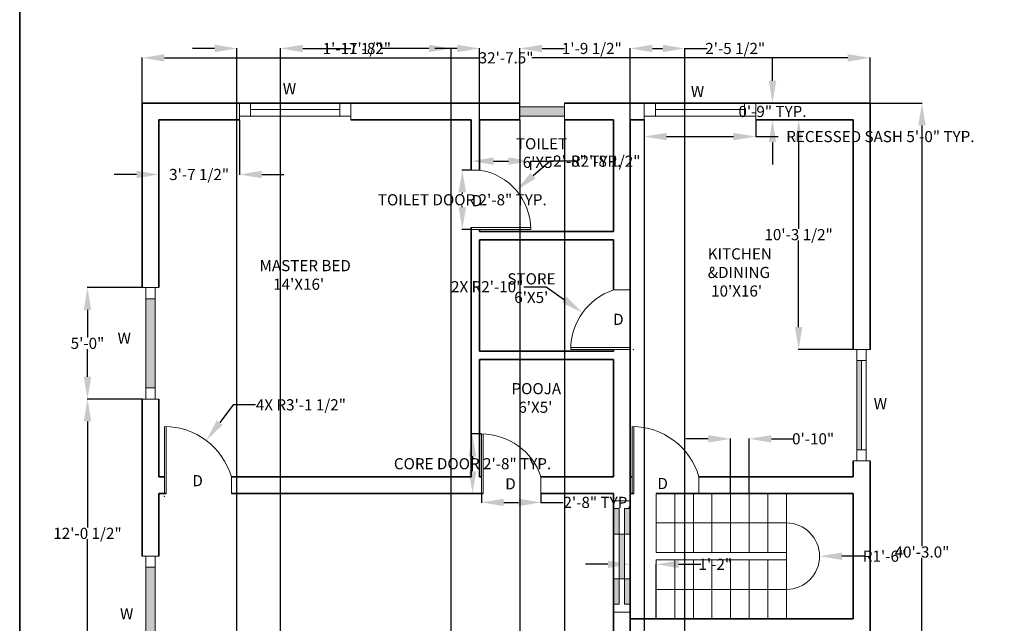
# Model space of a CAD drawing. Units: inches. Extents: x 115 to 1174, y 222 to 1302.
# Tile 2 of 5: x 115 to 644, y 521 to 846. Entities that reach past the tile are written whole.
import ezdxf

# ---------------------------------------------------------------- set-up
doc = ezdxf.new("R2010")
doc.units = ezdxf.units.IN
doc.header["$MEASUREMENT"] = 0
for name, color, linetype, lineweight in [('A-ANNO-DIMS', 2, 'Continuous', 18), ('A-ANNO-IDEN', 7, 'Continuous', 13), ('A-ANNO-TTLB', 7, 'Continuous', 35), ('A-AREA-IDEN', 7, 'Continuous', 18), ('A-DOOR', 3, 'Continuous', 18), ('A-FLOR-STRS', 7, 'Continuous', 18), ('A-GLAZ', 4, 'Continuous', 18), ('A-GLAZ-PATT', 8, 'Continuous', 13), ('A-WALL', 7, 'Continuous', 35)]:
    doc.layers.add(name, color=color, linetype=linetype, lineweight=lineweight)
doc.styles.get("Standard").update_dxf_attribs({"font": 'arial.ttf'})
doc.dimstyles.get("Standard").update_dxf_attribs({"dimtxt": 6, "dimasz": 12, "dimexe": 0.18, "dimexo": 0.0625, "dimgap": 0.09, "dimtad": 0, "dimtih": 1, "dimtoh": 1, "dimdec": 1, "dimzin": 0, "dimdsep": 46, "dimlunit": 3, "dimtxsty": 'Standard', "dimcen": 0.09, "dimadec": 0, "dimazin": 0, "dimtfac": 1, "dimtdec": 1, "dimtofl": 0, "dimtmove": 0, "dimatfit": 3, "dimfxl": 1, "dimtolj": 1, "dimtzin": 0, "dimarcsym": 0})

# ---------------------------------------------------------------- blocks, each defined once
blk = doc.blocks.new('*D1')
at = {"layer": 'A-ANNO-DIMS', "color": 0, "lineweight": -2, "transparency": 16777216}
for p, q in [((180.72, 801.13), (180.72, 825.59)), ((192.72, 825.41), (362.58, 825.41)), ((560.22, 825.41), (390.36, 825.41)), ((572.22, 801.13), (572.22, 825.59))]:
    blk.add_line(p, q, dxfattribs=at)
at = {"layer": 'A-ANNO-DIMS', "color": 0, "transparency": 16777216}
for points in [[(192.72, 827.41), (192.72, 823.41), (180.72, 825.41)], [(560.22, 827.41), (560.22, 823.41), (572.22, 825.41)]]:
    blk.add_solid(points, dxfattribs=at)
at = {"layer": 'Defpoints', "color": 0, "transparency": 16777216}
for p in [(572.22, 825.41), (180.72, 801.06), (572.22, 801.06)]:
    blk.add_point(p, dxfattribs=at)
at = {"layer": 'A-ANNO-DIMS', "color": 0, "transparency": 16777216, "insert": (376.47, 825.41), "char_height": 6, "attachment_point": 5}
blk.add_mtext('\\A1;32\'-7.5"', dxfattribs=at)
blk = doc.blocks.new('*D2')
at = {"layer": 'A-ANNO-DIMS', "color": 0, "lineweight": -2, "transparency": 16777216}
for p, q in [((572.28, 801.06), (600.35, 801.06)), ((600.17, 789.06), (600.17, 562.72)), ((600.17, 330.06), (600.17, 556.41)), ((572.28, 318.06), (600.35, 318.06))]:
    blk.add_line(p, q, dxfattribs=at)
at = {"layer": 'A-ANNO-DIMS', "color": 0, "transparency": 16777216}
for points in [[(598.17, 789.06), (602.17, 789.06), (600.17, 801.06)], [(598.17, 330.06), (602.17, 330.06), (600.17, 318.06)]]:
    blk.add_solid(points, dxfattribs=at)
at = {"layer": 'Defpoints', "color": 0, "transparency": 16777216}
for p in [(572.22, 801.06), (572.22, 318.06), (600.17, 318.06)]:
    blk.add_point(p, dxfattribs=at)
at = {"layer": 'A-ANNO-DIMS', "color": 0, "transparency": 16777216, "insert": (600.17, 559.56), "char_height": 6, "attachment_point": 5}
blk.add_mtext('\\A1;40\'-3.0"', dxfattribs=at)
blk = doc.blocks.new('DOOR-36-SWING')
for p, q in [((0, 0), (0, 36)), ((0, 36), (0, 0)), ((1, 36), (1, 0)), ((36, 0), (36, 9)), ((0, 0), (1, 0))]:
    blk.add_line(p, q)
blk.add_arc((0, -1.5), 37.5, 16.2602, 90)
blk = doc.blocks.new('DOOR-32-SWING')
for p, q in [((32, 32), (23, 32)), ((0, 1), (32, 1)), ((32, 0), (0, 0)), ((0, 0), (32, 0)), ((32, 0), (32, 1))]:
    blk.add_line(p, q)
blk.add_arc((33.76, 0), 33.76, 108.5866, 180)
blk = doc.blocks.new('DOOR-32-PARTITION')
for p, q in [((0, 32), (4.5, 32)), ((0, 0), (0, 1)), ((32, 1), (0, 1)), ((0, 0), (32, 0)), ((32, 0), (0, 0))]:
    blk.add_line(p, q)
blk.add_arc((-0.37, 0), 32.37, 0, 81.3499)
blk = doc.blocks.new('STAIR-HALF-TURN')
for p, q in [((0, 67.5), (0, 35.75)), ((10, 67.5), (10, 35.75)), ((20, 67.5), (20, 35.75)), ((30, 67.5), (30, 35.75)), ((40, 67.5), (40, 35.75)), ((50, 67.5), (50, 35.75)), ((60, 67.5), (60, 35.75)), ((70, 67.5), (70, 0)), ((106, 67.5), (106, 0)), ((0, 51.63), (70, 51.63)), ((70, 35.75), (0, 35.75)), ((70, 31.75), (0, 31.75)), ((0, 31.75), (0, 0)), ((10, 31.75), (10, 0)), ((20, 31.75), (20, 0)), ((30, 31.75), (30, 0)), ((40, 31.75), (40, 0)), ((50, 31.75), (50, 0)), ((60, 31.75), (60, 0)), ((0, 15.88), (70, 15.88))]:
    blk.add_line(p, q)
blk.add_arc((70, 33.75), 17.88, 270, 90)
blk = doc.blocks.new('WIN-60-RECESSED')
for p, q in [((0, 9), (0, 0)), ((60, 9), (0, 9)), ((6, 9), (6, 2)), ((6, 5.5), (54, 5.5)), ((54, 2), (54, 9)), ((60, 0), (60, 9)), ((0, 2), (60, 2))]:
    blk.add_line(p, q)
blk = doc.blocks.new('*D19')
at = {"layer": 'A-ANNO-DIMS', "color": 0, "lineweight": -2, "transparency": 16777216}
for p, q in [((363.16, 623.06), (358.24, 623.06)), ((358.42, 611.06), (358.42, 610.26)), ((358.42, 603.06), (358.42, 603.87)), ((363.16, 591.06), (358.24, 591.06))]:
    blk.add_line(p, q, dxfattribs=at)
at = {"layer": 'A-ANNO-DIMS', "color": 0, "transparency": 16777216}
for points in [[(356.42, 611.06), (360.42, 611.06), (358.42, 623.06)], [(356.42, 603.06), (360.42, 603.06), (358.42, 591.06)]]:
    blk.add_solid(points, dxfattribs=at)
at = {"layer": 'Defpoints', "color": 0, "transparency": 16777216}
for p in [(363.22, 623.06), (358.42, 591.06), (363.22, 591.06)]:
    blk.add_point(p, dxfattribs=at)
at = {"layer": 'A-ANNO-DIMS', "color": 0, "transparency": 16777216, "insert": (358.42, 607.06), "char_height": 6, "attachment_point": 5}
blk.add_mtext('\\A1;CORE DOOR 2\'-8" TYP.', dxfattribs=at)
blk = doc.blocks.new('*D20')
at = {"layer": 'A-ANNO-DIMS', "color": 0, "lineweight": -2, "transparency": 16777216}
for p, q in [((363.22, 591), (363.22, 586.08)), ((395.22, 591), (395.22, 586.08)), ((375.22, 586.26), (383.22, 586.26)), ((395.22, 586.26), (407.22, 586.26))]:
    blk.add_line(p, q, dxfattribs=at)
at = {"layer": 'A-ANNO-DIMS', "color": 0, "transparency": 16777216}
for points in [[(375.22, 588.26), (375.22, 584.26), (363.22, 586.26)], [(383.22, 588.26), (383.22, 584.26), (395.22, 586.26)]]:
    blk.add_solid(points, dxfattribs=at)
at = {"layer": 'Defpoints', "color": 0, "transparency": 16777216}
for p in [(363.22, 591.06), (395.22, 591.06), (395.22, 586.26)]:
    blk.add_point(p, dxfattribs=at)
at = {"layer": 'A-ANNO-DIMS', "color": 0, "transparency": 16777216, "insert": (425.65, 586.26), "char_height": 6, "attachment_point": 5}
blk.add_mtext('\\A1;2\'-8" TYP.', dxfattribs=at)
blk = doc.blocks.new('*D21')
at = {"layer": 'A-ANNO-DIMS', "color": 0, "lineweight": -2, "transparency": 16777216}
for p, q in [((357.66, 765.06), (352.74, 765.06)), ((352.92, 753.06), (352.92, 752.26)), ((352.92, 745.06), (352.92, 745.87)), ((357.66, 733.06), (352.74, 733.06))]:
    blk.add_line(p, q, dxfattribs=at)
at = {"layer": 'A-ANNO-DIMS', "color": 0, "transparency": 16777216}
for points in [[(350.92, 753.06), (354.92, 753.06), (352.92, 765.06)], [(350.92, 745.06), (354.92, 745.06), (352.92, 733.06)]]:
    blk.add_solid(points, dxfattribs=at)
at = {"layer": 'Defpoints', "color": 0, "transparency": 16777216}
for p in [(352.92, 765.06), (357.72, 765.06), (357.72, 733.06)]:
    blk.add_point(p, dxfattribs=at)
at = {"layer": 'A-ANNO-DIMS', "color": 0, "transparency": 16777216, "insert": (352.92, 749.06), "char_height": 6, "attachment_point": 5}
blk.add_mtext('\\A1;TOILET DOOR 2\'-8" TYP.', dxfattribs=at)
blk = doc.blocks.new('*D22')
at = {"layer": 'A-ANNO-DIMS', "color": 0, "lineweight": -2, "transparency": 16777216}
for p, q in [((357.72, 765.13), (357.72, 770.04)), ((369.72, 769.86), (377.72, 769.86)), ((389.72, 765.13), (389.72, 770.04)), ((389.72, 769.86), (401.72, 769.86))]:
    blk.add_line(p, q, dxfattribs=at)
at = {"layer": 'A-ANNO-DIMS', "color": 0, "transparency": 16777216}
for points in [[(369.72, 771.86), (369.72, 767.86), (357.72, 769.86)], [(377.72, 771.86), (377.72, 767.86), (389.72, 769.86)]]:
    blk.add_solid(points, dxfattribs=at)
at = {"layer": 'Defpoints', "color": 0, "transparency": 16777216}
for p in [(389.72, 769.86), (357.72, 765.06), (389.72, 765.06)]:
    blk.add_point(p, dxfattribs=at)
at = {"layer": 'A-ANNO-DIMS', "color": 0, "transparency": 16777216, "insert": (420.15, 769.86), "char_height": 6, "attachment_point": 5}
blk.add_mtext('\\A1;2\'-8" TYP.', dxfattribs=at)
blk = doc.blocks.new('*D25')
at = {"layer": 'A-ANNO-DIMS', "color": 0, "lineweight": -2, "transparency": 16777216}
for p, q in [((450.77, 792), (450.77, 782.88)), ((510.77, 792), (510.77, 782.88)), ((462.77, 783.06), (498.77, 783.06)), ((510.77, 783.06), (522.77, 783.06))]:
    blk.add_line(p, q, dxfattribs=at)
at = {"layer": 'A-ANNO-DIMS', "color": 0, "transparency": 16777216}
for points in [[(462.77, 785.06), (462.77, 781.06), (450.77, 783.06)], [(498.77, 785.06), (498.77, 781.06), (510.77, 783.06)]]:
    blk.add_solid(points, dxfattribs=at)
at = {"layer": 'Defpoints', "color": 0, "transparency": 16777216}
for p in [(450.77, 792.06), (510.77, 792.06), (510.77, 783.06)]:
    blk.add_point(p, dxfattribs=at)
at = {"layer": 'A-ANNO-DIMS', "color": 0, "transparency": 16777216, "insert": (577.79, 783.06), "char_height": 6, "attachment_point": 5}
blk.add_mtext('\\A1;RECESSED SASH 5\'-0" TYP.', dxfattribs=at)
blk = doc.blocks.new('*D26')
at = {"layer": 'A-ANNO-DIMS', "color": 0, "lineweight": -2, "transparency": 16777216}
for p, q in [((519.77, 813.06), (519.77, 825.06)), ((510.84, 801.06), (519.95, 801.06)), ((510.84, 792.06), (519.95, 792.06)), ((519.77, 780.06), (519.77, 768.06))]:
    blk.add_line(p, q, dxfattribs=at)
at = {"layer": 'A-ANNO-DIMS', "color": 0, "transparency": 16777216}
for points in [[(517.77, 813.06), (521.77, 813.06), (519.77, 801.06)], [(517.77, 780.06), (521.77, 780.06), (519.77, 792.06)]]:
    blk.add_solid(points, dxfattribs=at)
at = {"layer": 'Defpoints', "color": 0, "transparency": 16777216}
for p in [(510.77, 801.06), (519.77, 801.06), (510.77, 792.06)]:
    blk.add_point(p, dxfattribs=at)
at = {"layer": 'A-ANNO-DIMS', "color": 0, "transparency": 16777216, "insert": (519.77, 796.56), "char_height": 6, "attachment_point": 5}
blk.add_mtext('\\A1;0\'-9" TYP.', dxfattribs=at)
blk = doc.blocks.new('*D39')
at = {"layer": 'A-ANNO-DIMS', "color": 0, "lineweight": -2, "transparency": 16777216}
for p, q in [((180.66, 641.84), (151.14, 641.84)), ((151.32, 629.84), (151.32, 572.79)), ((151.32, 509.36), (151.32, 566.41)), ((180.66, 497.36), (151.14, 497.36))]:
    blk.add_line(p, q, dxfattribs=at)
at = {"layer": 'A-ANNO-DIMS', "color": 0, "transparency": 16777216}
for points in [[(149.32, 629.84), (153.32, 629.84), (151.32, 641.84)], [(149.32, 509.36), (153.32, 509.36), (151.32, 497.36)]]:
    blk.add_solid(points, dxfattribs=at)
at = {"layer": 'Defpoints', "color": 0, "transparency": 16777216}
for p in [(151.32, 641.84), (180.72, 641.84), (180.72, 497.36)]:
    blk.add_point(p, dxfattribs=at)
at = {"layer": 'A-ANNO-DIMS', "color": 0, "transparency": 16777216, "insert": (151.32, 569.6), "char_height": 6, "attachment_point": 5}
blk.add_mtext('\\A1;12\'-0 1/2"', dxfattribs=at)
blk = doc.blocks.new('*D40')
at = {"layer": 'A-ANNO-DIMS', "color": 0, "lineweight": -2, "transparency": 16777216}
for p, q in [((180.66, 701.84), (151.14, 701.84)), ((151.32, 689.84), (151.32, 674.99)), ((151.32, 653.84), (151.32, 668.68)), ((180.66, 641.84), (151.14, 641.84))]:
    blk.add_line(p, q, dxfattribs=at)
at = {"layer": 'A-ANNO-DIMS', "color": 0, "transparency": 16777216}
for points in [[(149.32, 689.84), (153.32, 689.84), (151.32, 701.84)], [(149.32, 653.84), (153.32, 653.84), (151.32, 641.84)]]:
    blk.add_solid(points, dxfattribs=at)
at = {"layer": 'Defpoints', "color": 0, "transparency": 16777216}
for p in [(151.32, 701.84), (180.72, 701.84), (180.72, 641.84)]:
    blk.add_point(p, dxfattribs=at)
at = {"layer": 'A-ANNO-DIMS', "color": 0, "transparency": 16777216, "insert": (151.32, 671.84), "char_height": 6, "attachment_point": 5}
blk.add_mtext('\\A1;5\'-0"', dxfattribs=at)
blk = doc.blocks.new('*D42')
at = {"layer": 'A-ANNO-DIMS', "color": 0, "lineweight": -2, "transparency": 16777216}
for p, q in [((563.16, 792.06), (533.64, 792.06)), ((533.82, 780.06), (533.82, 733.5)), ((533.82, 680.55), (533.82, 727.11)), ((563.16, 668.55), (533.64, 668.55))]:
    blk.add_line(p, q, dxfattribs=at)
at = {"layer": 'A-ANNO-DIMS', "color": 0, "transparency": 16777216}
for points in [[(531.82, 780.06), (535.82, 780.06), (533.82, 792.06)], [(531.82, 680.55), (535.82, 680.55), (533.82, 668.55)]]:
    blk.add_solid(points, dxfattribs=at)
at = {"layer": 'Defpoints', "color": 0, "transparency": 16777216}
for p in [(533.82, 792.06), (563.22, 792.06), (563.22, 668.55)]:
    blk.add_point(p, dxfattribs=at)
at = {"layer": 'A-ANNO-DIMS', "color": 0, "transparency": 16777216, "insert": (533.82, 730.31), "char_height": 6, "attachment_point": 5}
blk.add_mtext('\\A1;10\'-3 1/2"', dxfattribs=at)
blk = doc.blocks.new('*D43')
at = {"layer": 'A-ANNO-DIMS', "color": 0, "lineweight": -2, "transparency": 16777216}
for p, q in [((189.72, 792), (189.72, 762.48)), ((233.01, 792), (233.01, 762.48)), ((177.72, 762.66), (165.72, 762.66)), ((245.01, 762.66), (257.01, 762.66))]:
    blk.add_line(p, q, dxfattribs=at)
at = {"layer": 'A-ANNO-DIMS', "color": 0, "transparency": 16777216}
for points in [[(177.72, 764.66), (177.72, 760.66), (189.72, 762.66)], [(245.01, 764.66), (245.01, 760.66), (233.01, 762.66)]]:
    blk.add_solid(points, dxfattribs=at)
at = {"layer": 'Defpoints', "color": 0, "transparency": 16777216}
for p in [(189.72, 792.06), (233.01, 792.06), (189.72, 762.66)]:
    blk.add_point(p, dxfattribs=at)
at = {"layer": 'A-ANNO-DIMS', "color": 0, "transparency": 16777216, "insert": (211.36, 762.66), "char_height": 6, "attachment_point": 5}
blk.add_mtext('\\A1;3\'-7 1/2"', dxfattribs=at)
blk = doc.blocks.new('*D44')
at = {"layer": 'A-ANNO-DIMS', "color": 0, "lineweight": -2, "transparency": 16777216}
for p, q in [((350.22, 830.46), (338.22, 830.46)), ((362.22, 792.13), (362.22, 830.64)), ((383.83, 792.13), (383.83, 830.64)), ((395.83, 830.46), (407.83, 830.46))]:
    blk.add_line(p, q, dxfattribs=at)
at = {"layer": 'A-ANNO-DIMS', "color": 0, "transparency": 16777216}
for points in [[(350.22, 832.46), (350.22, 828.46), (362.22, 830.46)], [(395.83, 832.46), (395.83, 828.46), (383.83, 830.46)]]:
    blk.add_solid(points, dxfattribs=at)
at = {"layer": 'Defpoints', "color": 0, "transparency": 16777216}
for p in [(383.83, 830.46), (362.22, 792.06), (383.83, 792.06)]:
    blk.add_point(p, dxfattribs=at)
at = {"layer": 'A-ANNO-DIMS', "color": 0, "transparency": 16777216, "insert": (422.6, 830.46), "char_height": 6, "attachment_point": 5}
blk.add_mtext('\\A1;1\'-9 1/2"', dxfattribs=at)
blk = doc.blocks.new('*D45')
at = {"layer": 'A-ANNO-DIMS', "color": 0, "lineweight": -2, "transparency": 16777216}
for p, q in [((383.829365, 792.001973), (383.829365, 239.058512)), ((407.829365, 792.001973), (407.829365, 239.058512)), ((371.829365, 239.238512), (359.829365, 239.238512)), ((419.829365, 239.238512), (431.829365, 239.238512))]:
    blk.add_line(p, q, dxfattribs=at)
at = {"layer": 'A-ANNO-DIMS', "color": 0, "transparency": 16777216}
for points in [[(371.829365, 241.238512), (371.829365, 237.238512), (383.829365, 239.238512)], [(419.829365, 241.238512), (419.829365, 237.238512), (407.829365, 239.238512)]]:
    blk.add_solid(points, dxfattribs=at)
at = {"layer": 'Defpoints', "color": 0, "transparency": 16777216}
for p in [(383.829365, 792.064473), (407.829365, 792.064473), (407.829365, 239.238512)]:
    blk.add_point(p, dxfattribs=at)
at = {"layer": 'A-ANNO-DIMS', "color": 0, "transparency": 16777216, "insert": (395.829365, 239.238512), "char_height": 6, "attachment_point": 5}
blk.add_mtext('\\A1;2\'-0"', dxfattribs=at)
blk = doc.blocks.new('*D46')
at = {"layer": 'A-ANNO-DIMS', "color": 0, "lineweight": -2, "transparency": 16777216}
for p, q in [((443.22, 792), (443.22, 239.06)), ((450.77, 792), (450.77, 239.06)), ((431.22, 239.24), (419.22, 239.24)), ((462.77, 239.24), (474.77, 239.24))]:
    blk.add_line(p, q, dxfattribs=at)
at = {"layer": 'A-ANNO-DIMS', "color": 0, "transparency": 16777216}
for points in [[(431.22, 241.24), (431.22, 237.24), (443.22, 239.24)], [(462.77, 241.24), (462.77, 237.24), (450.77, 239.24)]]:
    blk.add_solid(points, dxfattribs=at)
at = {"layer": 'Defpoints', "color": 0, "transparency": 16777216}
for p in [(443.22, 792.06), (450.77, 792.06), (450.77, 239.24)]:
    blk.add_point(p, dxfattribs=at)
at = {"layer": 'A-ANNO-DIMS', "color": 0, "transparency": 16777216, "insert": (489.83, 239.24), "char_height": 6, "attachment_point": 5}
blk.add_mtext('\\A1;0\'-7 1/2"', dxfattribs=at)
blk = doc.blocks.new('*D48')
at = {"layer": 'A-ANNO-DIMS', "color": 0, "lineweight": -2, "transparency": 16777216}
for p, q in [((219.72, 830.46), (207.72, 830.46)), ((231.72, 327.13), (231.72, 830.64)), ((255.09, 327.13), (255.09, 830.64)), ((267.09, 830.46), (279.09, 830.46))]:
    blk.add_line(p, q, dxfattribs=at)
at = {"layer": 'A-ANNO-DIMS', "color": 0, "transparency": 16777216}
for points in [[(219.72, 832.46), (219.72, 828.46), (231.72, 830.46)], [(267.09, 832.46), (267.09, 828.46), (255.09, 830.46)]]:
    blk.add_solid(points, dxfattribs=at)
at = {"layer": 'Defpoints', "color": 0, "transparency": 16777216}
for p in [(255.09, 830.46), (231.72, 327.06), (255.09, 327.06)]:
    blk.add_point(p, dxfattribs=at)
at = {"layer": 'A-ANNO-DIMS', "color": 0, "transparency": 16777216, "insert": (296.19, 830.46), "char_height": 6, "attachment_point": 5}
blk.add_mtext('\\A1;1\'-11 1/2"', dxfattribs=at)
blk = doc.blocks.new('*D49')
at = {"layer": 'A-ANNO-DIMS', "color": 0, "lineweight": -2, "transparency": 16777216}
for p, q in [((255.09, 327.13), (255.09, 830.64)), ((267.09, 830.46), (292.98, 830.46)), ((334.96, 830.46), (309.06, 830.46)), ((346.96, 327.13), (346.96, 830.64))]:
    blk.add_line(p, q, dxfattribs=at)
at = {"layer": 'A-ANNO-DIMS', "color": 0, "transparency": 16777216}
for points in [[(267.09, 832.46), (267.09, 828.46), (255.09, 830.46)], [(334.96, 832.46), (334.96, 828.46), (346.96, 830.46)]]:
    blk.add_solid(points, dxfattribs=at)
at = {"layer": 'Defpoints', "color": 0, "transparency": 16777216}
for p in [(346.96, 830.46), (255.09, 327.06), (346.96, 327.06)]:
    blk.add_point(p, dxfattribs=at)
at = {"layer": 'A-ANNO-DIMS', "color": 0, "transparency": 16777216, "insert": (301.02, 830.46), "char_height": 6, "attachment_point": 5}
blk.add_mtext('\\A1;7\'-8"', dxfattribs=at)
blk = doc.blocks.new('*D50')
at = {"layer": 'A-ANNO-DIMS', "color": 0, "lineweight": -2, "transparency": 16777216}
for p, q in [((443.22, 327.13), (443.22, 830.64)), ((455.22, 830.46), (460.61, 830.46)), ((472.61, 327.13), (472.61, 830.64)), ((472.61, 830.46), (484.61, 830.46))]:
    blk.add_line(p, q, dxfattribs=at)
at = {"layer": 'A-ANNO-DIMS', "color": 0, "transparency": 16777216}
for points in [[(455.22, 832.46), (455.22, 828.46), (443.22, 830.46)], [(460.61, 832.46), (460.61, 828.46), (472.61, 830.46)]]:
    blk.add_solid(points, dxfattribs=at)
at = {"layer": 'Defpoints', "color": 0, "transparency": 16777216}
for p in [(472.61, 830.46), (443.22, 327.06), (472.61, 327.06)]:
    blk.add_point(p, dxfattribs=at)
at = {"layer": 'A-ANNO-DIMS', "color": 0, "transparency": 16777216, "insert": (499.71, 830.46), "char_height": 6, "attachment_point": 5}
blk.add_mtext('\\A1;2\'-5 1/2"', dxfattribs=at)
blk = doc.blocks.new('*D65')
at = {"layer": 'A-ANNO-DIMS', "color": 0, "lineweight": -2, "transparency": 16777216}
for p, q in [((431.22, 552.96), (419.22, 552.96)), ((443.22, 523.63), (443.22, 553.14)), ((457.22, 523.63), (457.22, 553.14)), ((469.22, 552.96), (481.22, 552.96))]:
    blk.add_line(p, q, dxfattribs=at)
at = {"layer": 'A-ANNO-DIMS', "color": 0, "transparency": 16777216}
for points in [[(431.22, 554.96), (431.22, 550.96), (443.22, 552.96)], [(469.22, 554.96), (469.22, 550.96), (457.22, 552.96)]]:
    blk.add_solid(points, dxfattribs=at)
at = {"layer": 'Defpoints', "color": 0, "transparency": 16777216}
for p in [(457.22, 552.96), (443.22, 523.56), (457.22, 523.56)]:
    blk.add_point(p, dxfattribs=at)
at = {"layer": 'A-ANNO-DIMS', "color": 0, "transparency": 16777216, "insert": (489, 552.96), "char_height": 6, "attachment_point": 5}
blk.add_mtext('\\A1;1\'-2"', dxfattribs=at)
blk = doc.blocks.new('*D66')
at = {"layer": 'A-ANNO-DIMS', "color": 0, "lineweight": -2, "transparency": 16777216}
for p, q in [((485.22, 620.46), (473.22, 620.46)), ((497.22, 591.13), (497.22, 620.64)), ((507.22, 591.13), (507.22, 620.64)), ((519.22, 620.46), (531.22, 620.46))]:
    blk.add_line(p, q, dxfattribs=at)
at = {"layer": 'A-ANNO-DIMS', "color": 0, "transparency": 16777216}
for points in [[(485.22, 622.46), (485.22, 618.46), (497.22, 620.46)], [(519.22, 622.46), (519.22, 618.46), (507.22, 620.46)]]:
    blk.add_solid(points, dxfattribs=at)
at = {"layer": 'Defpoints', "color": 0, "transparency": 16777216}
for p in [(507.22, 620.46), (497.22, 591.06), (507.22, 591.06)]:
    blk.add_point(p, dxfattribs=at)
at = {"layer": 'A-ANNO-DIMS', "color": 0, "transparency": 16777216, "insert": (541.62, 620.46), "char_height": 6, "attachment_point": 5}
blk.add_mtext('\\A1;0\'-10"', dxfattribs=at)
blk = doc.blocks.new('*D89')
at = {"layer": 'A-ANNO-DIMS', "color": 0, "lineweight": -2, "transparency": 16777216}
for p, q in [((229.62, 638.76), (222.42, 629.16)), ((241.62, 638.76), (229.62, 638.76)), ((192.63, 589.56), (192.81, 589.56)), ((192.72, 589.47), (192.72, 589.65))]:
    blk.add_line(p, q, dxfattribs=at)
at = {"layer": 'A-ANNO-DIMS', "color": 0, "transparency": 16777216}
blk.add_solid([(220.82, 630.36), (224.02, 627.96), (215.22, 619.56)], dxfattribs=at)
at = {"layer": 'Defpoints', "color": 0, "transparency": 16777216}
for p in [(215.22, 619.56), (192.72, 589.56)]:
    blk.add_point(p, dxfattribs=at)
at = {"layer": 'A-ANNO-DIMS', "color": 0, "transparency": 16777216, "insert": (266.11, 638.76), "char_height": 6, "attachment_point": 5}
blk.add_mtext('\\A1;4X R3\'-1 1/2"', dxfattribs=at)
blk = doc.blocks.new('*D90')
at = {"layer": 'A-ANNO-DIMS', "color": 0, "lineweight": -2, "transparency": 16777216}
for p, q in [((386.08, 702.28), (398.08, 702.28)), ((398.08, 702.28), (407.82, 695.27)), ((444.89, 668.56), (445.07, 668.56)), ((444.98, 668.47), (444.98, 668.65))]:
    blk.add_line(p, q, dxfattribs=at)
at = {"layer": 'A-ANNO-DIMS', "color": 0, "transparency": 16777216}
blk.add_solid([(408.99, 696.9), (406.65, 693.65), (417.57, 688.27)], dxfattribs=at)
at = {"layer": 'Defpoints', "color": 0, "transparency": 16777216}
for p in [(417.57, 688.27), (444.98, 668.56)]:
    blk.add_point(p, dxfattribs=at)
at = {"layer": 'A-ANNO-DIMS', "color": 0, "transparency": 16777216, "insert": (366.31, 702.28), "char_height": 6, "attachment_point": 5}
blk.add_mtext('\\A1;2X R2\'-10"', dxfattribs=at)
blk = doc.blocks.new('*D91')
at = {"layer": 'A-ANNO-DIMS', "color": 0, "lineweight": -2, "transparency": 16777216}
for p, q in [((400.1, 769.8), (391, 761.98)), ((412.1, 769.8), (400.1, 769.8)), ((357.26, 733.06), (357.44, 733.06)), ((357.35, 732.97), (357.35, 733.15))]:
    blk.add_line(p, q, dxfattribs=at)
at = {"layer": 'A-ANNO-DIMS', "color": 0, "transparency": 16777216}
blk.add_solid([(389.7, 763.5), (392.3, 760.47), (381.9, 754.16)], dxfattribs=at)
at = {"layer": 'Defpoints', "color": 0, "transparency": 16777216}
for p in [(381.9, 754.16), (357.35, 733.06)]:
    blk.add_point(p, dxfattribs=at)
at = {"layer": 'A-ANNO-DIMS', "color": 0, "transparency": 16777216, "insert": (430.03, 769.8), "char_height": 6, "attachment_point": 5}
blk.add_mtext('\\A1;R2\'-8 1/2"', dxfattribs=at)
blk = doc.blocks.new('*D92')
at = {"layer": 'A-ANNO-DIMS', "color": 0, "lineweight": -2, "transparency": 16777216}
for p, q in [((527.13, 557.31), (527.31, 557.31)), ((527.22, 557.22), (527.22, 557.4)), ((569.09, 557.31), (557.09, 557.31))]:
    blk.add_line(p, q, dxfattribs=at)
at = {"layer": 'A-ANNO-DIMS', "color": 0, "transparency": 16777216}
blk.add_solid([(557.09, 559.31), (557.09, 555.31), (545.09, 557.31)], dxfattribs=at)
at = {"layer": 'Defpoints', "color": 0, "transparency": 16777216}
for p in [(527.22, 557.31), (545.09, 557.31)]:
    blk.add_point(p, dxfattribs=at)
at = {"layer": 'A-ANNO-DIMS', "color": 0, "transparency": 16777216, "insert": (580.03, 557.31), "char_height": 6, "attachment_point": 5}
blk.add_mtext('\\A1;R1\'-6"', dxfattribs=at)

msp = doc.modelspace()

# ---------------------------------------------------------------- hatches: boundary and pattern name
at = {"layer": 'A-GLAZ-PATT'}
h = msp.add_hatch(color=256, dxfattribs=at)
h.dxf.hatch_style = 1
h.paths.add_polyline_path([(407.83, 799.06), (383.83, 799.06), (383.83, 794.06), (407.83, 794.06)])
h.paths.add_polyline_path([(567.72, 662.55), (565.22, 662.55), (565.22, 614.55), (567.72, 614.55)])
h.paths.add_polyline_path([(567.72, 435.27), (565.22, 435.27), (565.22, 387.27), (567.72, 387.27)])
h.paths.add_polyline_path([(187.72, 444.28), (182.72, 444.28), (182.72, 396.28), (187.72, 396.28)])
h.paths.add_polyline_path([(187.72, 551.36), (182.72, 551.36), (182.72, 503.36), (187.72, 503.36)])
h.paths.add_polyline_path([(187.72, 695.84), (182.72, 695.84), (182.72, 647.84), (187.72, 647.84)])
h = msp.add_hatch(color=256, dxfattribs=at)
h.dxf.hatch_style = 1
h.paths.add_polyline_path([(443.22, 582.97), (440.22, 582.97), (440.22, 569.22), (443.22, 569.22)])
h.paths.add_polyline_path([(437.22, 582.97), (434.22, 582.97), (434.22, 569.22), (437.22, 569.22)])
h.paths.add_polyline_path([(440.22, 569.22), (437.22, 569.22), (437.22, 545.22), (440.22, 545.22)])
h.paths.add_polyline_path([(443.22, 545.22), (440.22, 545.22), (440.22, 531.52), (443.22, 531.52)])
h.paths.add_polyline_path([(437.22, 545.22), (434.22, 545.22), (434.22, 531.52), (437.22, 531.52)])

# ---------------------------------------------------------------- linework, layer by layer
at = {"layer": 'A-ANNO-TTLB'}
msp.add_lwpolyline([(114.85, 1302.15), (1174.06, 1302.15), (1174.06, 222.13), (114.85, 222.13)], close=True, dxfattribs=at)
at = {"layer": 'A-GLAZ'}
for p, q in [((383.83, 801.06), (383.83, 792.06)), ((407.83, 792.06), (407.83, 801.06)), ((407.83, 799.06), (383.83, 799.06)), ((383.83, 794.06), (407.83, 794.06)), ((180.72, 701.84), (189.72, 701.84)), ((182.72, 641.84), (182.72, 701.84)), ((187.72, 701.84), (187.72, 641.84)), ((182.72, 695.84), (187.72, 695.84)), ((563.22, 668.55), (572.22, 668.55)), ((565.22, 608.55), (565.22, 668.55)), ((570.22, 668.55), (570.22, 608.55)), ((565.22, 662.55), (570.22, 662.55)), ((567.72, 662.55), (567.72, 614.55)), ((187.72, 647.84), (182.72, 647.84)), ((189.72, 641.84), (180.72, 641.84)), ((570.22, 614.55), (565.22, 614.55)), ((572.22, 608.55), (563.22, 608.55)), ((443.22, 587.16), (434.22, 587.16)), ((434.22, 587.16), (434.22, 527.29)), ((434.22, 582.97), (437.22, 582.97)), ((437.22, 582.97), (437.22, 531.52)), ((440.22, 531.52), (440.22, 582.97)), ((440.22, 582.97), (443.22, 582.97)), ((443.22, 527.29), (443.22, 587.16)), ((443.22, 569.22), (434.22, 569.22)), ((180.72, 557.36), (189.72, 557.36)), ((182.72, 497.36), (182.72, 557.36)), ((187.72, 557.36), (187.72, 497.36)), ((182.72, 551.36), (187.72, 551.36)), ((443.22, 545.22), (434.22, 545.22)), ((434.22, 527.29), (434.22, 531.52)), ((434.22, 531.52), (437.22, 531.52)), ((440.22, 531.52), (443.22, 531.52)), ((443.22, 531.52), (443.22, 527.29)), ((434.22, 527.29), (443.22, 527.29))]:
    msp.add_line(p, q, dxfattribs=at)
at = {"layer": 'A-WALL'}
for p, q in [((180.72, 801.06), (383.83, 801.06)), ((180.72, 801.06), (180.72, 701.84)), ((407.83, 801.06), (572.22, 801.06)), ((572.22, 801.06), (572.22, 668.55)), ((189.72, 792.06), (189.72, 701.84)), ((189.72, 792.06), (233.01, 792.06)), ((293.01, 792.06), (357.72, 792.06)), ((357.72, 792.06), (357.72, 765.06)), ((362.22, 792.06), (362.22, 765.06)), ((362.22, 792.06), (383.83, 792.06)), ((407.83, 792.06), (434.22, 792.06)), ((434.22, 792.06), (434.22, 732.06)), ((443.22, 792.06), (443.22, 700.56)), ((443.22, 792.06), (450.77, 792.06)), ((510.77, 792.06), (563.22, 792.06)), ((563.22, 792.06), (563.22, 668.55)), ((357.72, 734.06), (357.72, 600.06)), ((357.72, 732.06), (357.72, 733.06)), ((362.22, 733.06), (362.22, 732.06)), ((362.22, 732.06), (434.22, 732.06)), ((362.22, 727.56), (434.22, 727.56)), ((362.22, 727.56), (362.22, 667.56)), ((434.22, 727.56), (434.22, 700.56)), ((362.22, 667.56), (434.22, 667.56)), ((434.22, 668.56), (434.22, 667.56)), ((443.22, 669.56), (443.22, 600.06)), ((443.22, 667.56), (443.22, 668.56)), ((362.22, 663.06), (434.22, 663.06)), ((362.22, 663.06), (362.22, 600.06)), ((434.22, 663.06), (434.22, 600.06)), ((180.72, 641.84), (180.72, 557.36)), ((189.72, 641.84), (189.72, 600.06)), ((563.22, 608.55), (563.22, 600.06)), ((572.22, 608.55), (572.22, 441.27)), ((189.72, 600.06), (192.72, 600.06)), ((228.72, 600.06), (357.72, 600.06)), ((362.22, 600.06), (363.22, 600.06)), ((395.22, 600.06), (434.22, 600.06)), ((443.22, 600.06), (444.22, 600.06)), ((480.22, 600.06), (563.22, 600.06)), ((189.72, 591.06), (193.72, 591.06)), ((189.72, 591.06), (192.72, 591.06)), ((189.72, 591.06), (189.72, 557.36)), ((228.72, 591.06), (364.22, 591.06)), ((362.22, 591.06), (363.22, 591.06)), ((395.22, 591.06), (434.22, 591.06)), ((434.22, 591.06), (434.22, 512.06)), ((443.22, 591.06), (444.22, 591.06)), ((443.22, 591.06), (443.22, 523.56)), ((443.22, 591.06), (445.22, 591.06)), ((457.22, 591.06), (563.22, 591.06)), ((563.22, 591.06), (563.22, 523.56)), ((443.22, 523.56), (563.22, 523.56))]:
    msp.add_line(p, q, dxfattribs=at)

# ---------------------------------------------------------------- block references
at = {"layer": 'A-DOOR'}
for name, p in [('DOOR-32-PARTITION', (357.72, 733.06)), ('DOOR-32-SWING', (411.22, 668.56)), ('DOOR-36-SWING', (192.72, 591.06)), ('DOOR-36-SWING', (444.22, 591.06))]:
    msp.add_blockref(name, p, dxfattribs=at)
at = {"layer": 'A-DOOR', "rotation": 269.9999999999998}
msp.add_blockref('DOOR-32-SWING', (363.22, 623.06), dxfattribs=at)
at = {"layer": 'A-FLOR-STRS'}
msp.add_blockref('STAIR-HALF-TURN', (457.22, 523.56), dxfattribs=at)
at = {"layer": 'A-GLAZ'}
for p in [(233.01, 792.06), (450.77, 792.06)]:
    msp.add_blockref('WIN-60-RECESSED', p, dxfattribs=at)

# ---------------------------------------------------------------- texts
at = {"layer": 'A-ANNO-IDEN', "char_height": 6, "attachment_point": 1}
for s, width, heights, insert in [('W', 10.5593, [0], (256.38, 811.79)), ('W', 10.5593, [0], (475.85, 810.35)), ('D', 9.3758, [0], (357.98, 751.6)), ('D', 9.3758, [0], (434.08, 687.72)), ('W', 9.7663, [6], (167.5, 677.59)), ('W', 10.5593, [0], (574.21, 642.36)), ('D', 9.3758, [0], (207.74, 600.94)), ('D', 9.3758, [0], (376.04, 599.27)), ('D', 9.3758, [0], (457.88, 599.42)), ('W', 10.5593, [0], (168.81, 529.36))]:
    msp.add_mtext_dynamic_manual_height_columns(s, width=width, gutter_width=30, heights=heights, dxfattribs=dict(at, insert=insert))
at = {"layer": 'A-AREA-IDEN', "char_height": 6, "attachment_point": 1}
for s, width, insert in [("TOILET\\P  6'X5'", 41.5684, (381.76, 782.2)), ("KITCHEN\\P&DINING\\P 10'X16'", 70.6782, (484.94, 722.97)), ("MASTER BED\\P    14'X16'", 61.0364, (243.88, 716.64)), ("STORE\\P  6'X5'", 36.104, (377.2, 709.52)), ("POOJA\\P  6'X5'", 44.1433, (379.39, 650.45))]:
    msp.add_mtext_dynamic_manual_height_columns(s, width=width, gutter_width=30, heights=[0], dxfattribs=dict(at, insert=insert))

# ---------------------------------------------------------------- dimensions: what is measured, and where the dimension line sits
at = {"layer": 'A-ANNO-DIMS'}
for base, p1, p2, override, picture, middle in [((255.09, 830.46), (231.72, 327.06), (255.09, 327.06), {"dimdec": 1, "dimlfac": 1, "dimrnd": 0, "dimzin": 1, "dimdsep": 46, "dimlunit": 4, "dimfrac": 2}, '*D48', (296.19, 830.46)), ((383.83, 830.46), (362.22, 792.06), (383.83, 792.06), {"dimdec": 1, "dimlfac": 1, "dimrnd": 0, "dimzin": 1, "dimdsep": 46, "dimlunit": 4, "dimfrac": 2}, '*D44', (422.6, 830.46)), ((472.61, 830.46), (443.22, 327.06), (472.61, 327.06), {"dimdec": 1, "dimlfac": 1, "dimrnd": 0, "dimzin": 1, "dimdsep": 46, "dimlunit": 4, "dimfrac": 2}, '*D50', (499.71, 830.46)), ((346.96, 830.46), (255.09, 327.06), (346.96, 327.06), {"dimdec": 1, "dimlfac": 1, "dimrnd": 0, "dimzin": 1, "dimdsep": 46, "dimlunit": 4, "dimfrac": 2}, '*D49', (301.02, 830.46)), ((572.22, 825.41), (180.72, 801.06), (572.22, 801.06), {"dimclrd": 0, "dimclre": 0, "dimclrt": 0}, '*D1', (376.47, 825.41)), ((407.83, 239.24), (383.83, 792.06), (407.83, 792.06), {"dimdec": 1, "dimlfac": 1, "dimrnd": 0, "dimzin": 1, "dimdsep": 46, "dimlunit": 4, "dimfrac": 2}, '*D45', (395.83, 239.24)), ((450.7739, 239.2385), (443.2197, 792.0645), (450.7739, 792.0645), {"dimdec": 1, "dimlfac": 1, "dimrnd": 0, "dimzin": 1, "dimdsep": 46, "dimlunit": 4, "dimfrac": 2}, '*D46', (489.8291, 239.2385)), ((507.22, 620.46), (497.22, 591.06), (507.22, 591.06), {"dimdec": 1, "dimlfac": 1, "dimrnd": 0, "dimzin": 1, "dimdsep": 46, "dimlunit": 4, "dimfrac": 2}, '*D66', (541.62, 620.46)), ((457.22, 552.96), (443.22, 523.56), (457.22, 523.56), {"dimdec": 1, "dimlfac": 1, "dimrnd": 0, "dimzin": 1, "dimdsep": 46, "dimlunit": 4, "dimfrac": 2}, '*D65', (489, 552.96))]:
    dim = msp.add_linear_dim(base=base, p1=p1, p2=p2, dimstyle='Standard', override=override, dxfattribs=at)
    dim.commit()
    dim.dimension.update_dxf_attribs({"geometry": picture, "text_midpoint": middle})
for base, p1, p2, angle, text, picture, middle in [((519.77, 801.06), (510.77, 792.06), (510.77, 801.06), 90, '<> TYP.', '*D26', (519.77, 796.56)), ((352.92, 765.06), (357.72, 733.06), (357.72, 765.06), 90, 'TOILET DOOR <> TYP.', '*D21', (352.92, 749.06)), ((358.42, 591.06), (363.22, 623.06), (363.22, 591.06), 270, 'CORE DOOR <> TYP.', '*D19', (358.42, 607.06))]:
    dim = msp.add_linear_dim(base=base, p1=p1, p2=p2, angle=angle, text=text, dimstyle='Standard', override={"dimdec": 1, "dimlfac": 1, "dimrnd": 0, "dimzin": 1, "dimdsep": 46, "dimlunit": 4, "dimfrac": 2}, dxfattribs=at)
    dim.commit()
    dim.dimension.update_dxf_attribs({"geometry": picture, "text_midpoint": middle})
for base, p1, p2, text, picture, middle in [((510.77, 783.06), (450.77, 792.06), (510.77, 792.06), 'RECESSED SASH <> TYP.', '*D25', (577.79, 783.06)), ((389.72, 769.86), (357.72, 765.06), (389.72, 765.06), '<> TYP.', '*D22', (420.15, 769.86)), ((395.22, 586.26), (363.22, 591.06), (395.22, 591.06), '<> TYP.', '*D20', (425.65, 586.26))]:
    dim = msp.add_linear_dim(base=base, p1=p1, p2=p2, text=text, dimstyle='Standard', override={"dimdec": 1, "dimlfac": 1, "dimrnd": 0, "dimzin": 1, "dimdsep": 46, "dimlunit": 4, "dimfrac": 2}, dxfattribs=at)
    dim.commit()
    dim.dimension.update_dxf_attribs({"geometry": picture, "text_midpoint": middle})
for base, p1, p2, angle, override, picture, middle in [((600.17, 318.06), (572.22, 801.06), (572.22, 318.06), 90, {"dimclrd": 0, "dimclre": 0, "dimclrt": 0}, '*D2', (600.17, 559.56)), ((189.72, 762.66), (233.01, 792.06), (189.72, 792.06), 180, {"dimdec": 1, "dimlfac": 1, "dimrnd": 0, "dimzin": 1, "dimdsep": 46, "dimlunit": 4, "dimfrac": 2}, '*D43', (211.36, 762.66)), ((533.82, 792.06), (563.22, 668.55), (563.22, 792.06), 90, {"dimdec": 1, "dimlfac": 1, "dimrnd": 0, "dimzin": 1, "dimdsep": 46, "dimlunit": 4, "dimfrac": 2}, '*D42', (533.82, 730.31)), ((151.32, 701.84), (180.72, 641.84), (180.72, 701.84), 90, {"dimdec": 1, "dimlfac": 1, "dimrnd": 0, "dimzin": 1, "dimdsep": 46, "dimlunit": 4, "dimfrac": 2}, '*D40', (151.32, 671.84)), ((151.32, 641.84), (180.72, 497.36), (180.72, 641.84), 90, {"dimdec": 1, "dimlfac": 1, "dimrnd": 0, "dimzin": 1, "dimdsep": 46, "dimlunit": 4, "dimfrac": 2}, '*D39', (151.32, 569.6))]:
    dim = msp.add_linear_dim(base=base, p1=p1, p2=p2, angle=angle, dimstyle='Standard', override=override, dxfattribs=at)
    dim.commit()
    dim.dimension.update_dxf_attribs({"geometry": picture, "text_midpoint": middle})
for center, mpoint, picture, middle in [((357.35, 733.06), (381.9, 754.16), '*D91', (430.03, 769.8)), ((527.22, 557.31), (545.09, 557.31), '*D92', (580.03, 557.31))]:
    dim = msp.add_radius_dim(center=center, mpoint=mpoint, dimstyle='Standard', override={"dimdec": 1, "dimlfac": 1, "dimrnd": 0, "dimzin": 1, "dimdsep": 46, "dimlunit": 4, "dimfrac": 2}, dxfattribs=at)
    dim.commit()
    dim.dimension.update_dxf_attribs({"geometry": picture, "text_midpoint": middle})
for center, mpoint, text, picture, middle in [((444.98, 668.56), (417.57, 688.27), '2X <>', '*D90', (366.31, 702.28)), ((192.72, 589.56), (215.22, 619.56), '4X <>', '*D89', (266.11, 638.76))]:
    dim = msp.add_radius_dim(center=center, mpoint=mpoint, text=text, dimstyle='Standard', override={"dimdec": 1, "dimlfac": 1, "dimrnd": 0, "dimzin": 1, "dimdsep": 46, "dimlunit": 4, "dimfrac": 2}, dxfattribs=at)
    dim.commit()
    dim.dimension.update_dxf_attribs({"geometry": picture, "text_midpoint": middle})

doc.saveas('drawing.dxf')
